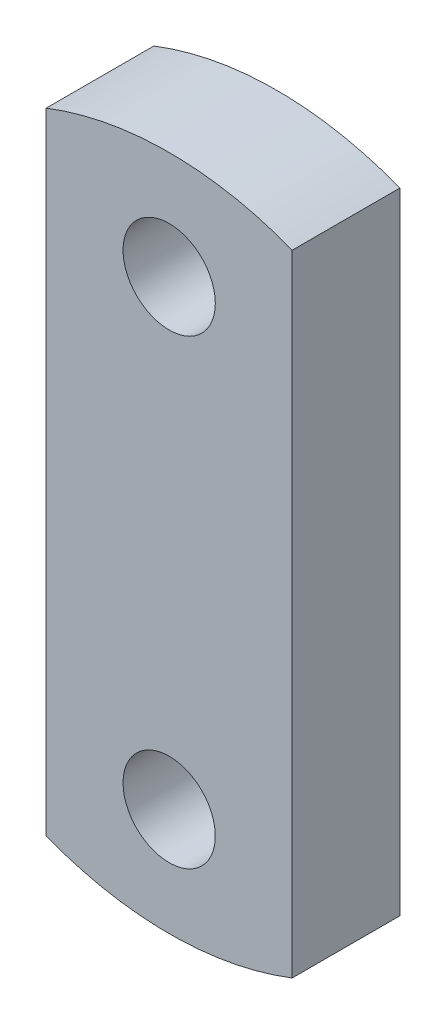
ISO-10303-21;
HEADER;
FILE_DESCRIPTION(('STEP AP214'),'2;1');
FILE_NAME('part.step','',(''),(''),'','','');
FILE_SCHEMA(('AUTOMOTIVE_DESIGN { 1 0 10303 214 1 1 1 1 }'));
ENDSEC;
DATA;
#1=APPLICATION_CONTEXT('core data for automotive mechanical design processes');
#2=APPLICATION_PROTOCOL_DEFINITION('international standard','automotive_design',2000,#1);
#3=PRODUCT_CONTEXT('',#1,'mechanical');
#4=PRODUCT('Part','Part','',(#3));
#5=PRODUCT_RELATED_PRODUCT_CATEGORY('part','',(#4));
#6=PRODUCT_DEFINITION_FORMATION('','',#4);
#7=PRODUCT_DEFINITION_CONTEXT('part definition',#1,'design');
#8=PRODUCT_DEFINITION('design','',#6,#7);
#9=PRODUCT_DEFINITION_SHAPE('','',#8);
#10=(LENGTH_UNIT() NAMED_UNIT(*) SI_UNIT(.MILLI.,.METRE.));
#11=(NAMED_UNIT(*) PLANE_ANGLE_UNIT() SI_UNIT($,.RADIAN.));
#12=(NAMED_UNIT(*) SI_UNIT($,.STERADIAN.) SOLID_ANGLE_UNIT());
#13=UNCERTAINTY_MEASURE_WITH_UNIT(LENGTH_MEASURE(1.E-05),#10,'distance_accuracy_value','');
#14=(GEOMETRIC_REPRESENTATION_CONTEXT(3) GLOBAL_UNCERTAINTY_ASSIGNED_CONTEXT((#13)) GLOBAL_UNIT_ASSIGNED_CONTEXT((#10,
#11,#12)) REPRESENTATION_CONTEXT('',''));
#15=CARTESIAN_POINT('',(0.,0.,0.));
#16=DIRECTION('',(0.,0.,1.));
#17=DIRECTION('',(1.,0.,0.));
#18=AXIS2_PLACEMENT_3D('',#15,#16,#17);
#19=CARTESIAN_POINT('',(0.,0.,17.5));
#20=DIRECTION('',(0.,0.,-1.));
#21=DIRECTION('',(-1.,0.,0.));
#22=AXIS2_PLACEMENT_3D('',#19,#20,#21);
#23=PLANE('',#22);
#24=CARTESIAN_POINT('',(0.,0.,17.5));
#25=DIRECTION('',(0.,0.,1.));
#26=DIRECTION('',(-1.,0.,0.));
#27=AXIS2_PLACEMENT_3D('',#24,#25,#26);
#28=CIRCLE('',#27,110.);
#29=CARTESIAN_POINT('',(40.,102.469507659596,17.5));
#30=VERTEX_POINT('',#29);
#31=CARTESIAN_POINT('',(-40.,102.469507659596,17.5));
#32=VERTEX_POINT('',#31);
#33=EDGE_CURVE('E93',#30,#32,#28,.T.);
#34=ORIENTED_EDGE('',*,*,#33,.T.);
#35=DIRECTION('',(0.,-1.,0.));
#36=VECTOR('',#35,1.);
#37=CARTESIAN_POINT('',(-40.,-102.469507659596,17.5));
#38=LINE('',#37,#36);
#39=CARTESIAN_POINT('',(-40.,-102.469507659596,17.5));
#40=VERTEX_POINT('',#39);
#41=EDGE_CURVE('E88',#32,#40,#38,.T.);
#42=ORIENTED_EDGE('',*,*,#41,.T.);
#43=CARTESIAN_POINT('',(0.,0.,17.5));
#44=DIRECTION('',(0.,0.,1.));
#45=DIRECTION('',(1.,0.,0.));
#46=AXIS2_PLACEMENT_3D('',#43,#44,#45);
#47=CIRCLE('',#46,110.);
#48=CARTESIAN_POINT('',(40.,-102.469507659596,17.5));
#49=VERTEX_POINT('',#48);
#50=EDGE_CURVE('E90',#40,#49,#47,.T.);
#51=ORIENTED_EDGE('',*,*,#50,.T.);
#52=DIRECTION('',(0.,1.,0.));
#53=VECTOR('',#52,1.);
#54=CARTESIAN_POINT('',(40.,-102.469507659596,17.5));
#55=LINE('',#54,#53);
#56=EDGE_CURVE('E57',#49,#30,#55,.T.);
#57=ORIENTED_EDGE('',*,*,#56,.T.);
#58=EDGE_LOOP('',(#34,#42,#51,#57));
#59=FACE_BOUND('',#58,.T.);
#60=CARTESIAN_POINT('',(0.,75.,17.5));
#61=DIRECTION('',(0.,0.,1.));
#62=DIRECTION('',(1.,0.,0.));
#63=AXIS2_PLACEMENT_3D('',#60,#61,#62);
#64=CIRCLE('',#63,15.);
#65=CARTESIAN_POINT('',(15.,75.,17.5));
#66=VERTEX_POINT('',#65);
#67=EDGE_CURVE('E106',#66,#66,#64,.T.);
#68=ORIENTED_EDGE('',*,*,#67,.F.);
#69=EDGE_LOOP('',(#68));
#70=FACE_BOUND('',#69,.T.);
#71=CARTESIAN_POINT('',(0.,-75.,17.5));
#72=DIRECTION('',(0.,0.,1.));
#73=DIRECTION('',(-1.,0.,0.));
#74=AXIS2_PLACEMENT_3D('',#71,#72,#73);
#75=CIRCLE('',#74,15.);
#76=CARTESIAN_POINT('',(-15.,-75.,17.5));
#77=VERTEX_POINT('',#76);
#78=EDGE_CURVE('E121',#77,#77,#75,.T.);
#79=ORIENTED_EDGE('',*,*,#78,.F.);
#80=EDGE_LOOP('',(#79));
#81=FACE_BOUND('',#80,.T.);
#82=ADVANCED_FACE('F39',(#59,#70,#81),#23,.F.);
#83=CARTESIAN_POINT('',(0.,0.,-17.5));
#84=DIRECTION('',(0.,0.,-1.));
#85=DIRECTION('',(-1.,0.,0.));
#86=AXIS2_PLACEMENT_3D('',#83,#84,#85);
#87=PLANE('',#86);
#88=CARTESIAN_POINT('',(0.,75.,-17.5));
#89=DIRECTION('',(0.,0.,1.));
#90=DIRECTION('',(1.,0.,0.));
#91=AXIS2_PLACEMENT_3D('',#88,#89,#90);
#92=CIRCLE('',#91,15.);
#93=CARTESIAN_POINT('',(15.,75.,-17.5));
#94=VERTEX_POINT('',#93);
#95=EDGE_CURVE('E119',#94,#94,#92,.T.);
#96=ORIENTED_EDGE('',*,*,#95,.T.);
#97=EDGE_LOOP('',(#96));
#98=FACE_BOUND('',#97,.T.);
#99=CARTESIAN_POINT('',(0.,0.,-17.5));
#100=DIRECTION('',(0.,0.,1.));
#101=DIRECTION('',(-1.,0.,0.));
#102=AXIS2_PLACEMENT_3D('',#99,#100,#101);
#103=CIRCLE('',#102,110.);
#104=CARTESIAN_POINT('',(40.,102.469507659596,-17.5));
#105=VERTEX_POINT('',#104);
#106=CARTESIAN_POINT('',(-40.,102.469507659596,-17.5));
#107=VERTEX_POINT('',#106);
#108=EDGE_CURVE('E103',#105,#107,#103,.T.);
#109=ORIENTED_EDGE('',*,*,#108,.F.);
#110=DIRECTION('',(0.,1.,0.));
#111=VECTOR('',#110,1.);
#112=CARTESIAN_POINT('',(40.,-102.469507659596,-17.5));
#113=LINE('',#112,#111);
#114=CARTESIAN_POINT('',(40.,-102.469507659596,-17.5));
#115=VERTEX_POINT('',#114);
#116=EDGE_CURVE('E76',#115,#105,#113,.T.);
#117=ORIENTED_EDGE('',*,*,#116,.F.);
#118=CARTESIAN_POINT('',(0.,0.,-17.5));
#119=DIRECTION('',(0.,0.,1.));
#120=DIRECTION('',(1.,0.,0.));
#121=AXIS2_PLACEMENT_3D('',#118,#119,#120);
#122=CIRCLE('',#121,110.);
#123=CARTESIAN_POINT('',(-40.,-102.469507659596,-17.5));
#124=VERTEX_POINT('',#123);
#125=EDGE_CURVE('E71',#124,#115,#122,.T.);
#126=ORIENTED_EDGE('',*,*,#125,.F.);
#127=DIRECTION('',(0.,-1.,0.));
#128=VECTOR('',#127,1.);
#129=CARTESIAN_POINT('',(-40.,-102.469507659596,-17.5));
#130=LINE('',#129,#128);
#131=EDGE_CURVE('E92',#107,#124,#130,.T.);
#132=ORIENTED_EDGE('',*,*,#131,.F.);
#133=EDGE_LOOP('',(#109,#117,#126,#132));
#134=FACE_BOUND('',#133,.T.);
#135=CARTESIAN_POINT('',(0.,-75.,-17.5));
#136=DIRECTION('',(0.,0.,1.));
#137=DIRECTION('',(-1.,0.,0.));
#138=AXIS2_PLACEMENT_3D('',#135,#136,#137);
#139=CIRCLE('',#138,15.);
#140=CARTESIAN_POINT('',(-15.,-75.,-17.5));
#141=VERTEX_POINT('',#140);
#142=EDGE_CURVE('E122',#141,#141,#139,.T.);
#143=ORIENTED_EDGE('',*,*,#142,.T.);
#144=EDGE_LOOP('',(#143));
#145=FACE_BOUND('',#144,.T.);
#146=ADVANCED_FACE('F111',(#98,#134,#145),#87,.T.);
#147=CARTESIAN_POINT('',(0.,0.,17.5));
#148=DIRECTION('',(0.,0.,-1.));
#149=DIRECTION('',(-1.,0.,0.));
#150=AXIS2_PLACEMENT_3D('',#147,#148,#149);
#151=CYLINDRICAL_SURFACE('',#150,110.);
#152=ORIENTED_EDGE('',*,*,#108,.T.);
#153=DIRECTION('',(0.,0.,-1.));
#154=VECTOR('',#153,1.);
#155=CARTESIAN_POINT('',(-40.,102.469507659596,17.5));
#156=LINE('',#155,#154);
#157=EDGE_CURVE('E11',#32,#107,#156,.T.);
#158=ORIENTED_EDGE('',*,*,#157,.F.);
#159=ORIENTED_EDGE('',*,*,#33,.F.);
#160=DIRECTION('',(0.,0.,-1.));
#161=VECTOR('',#160,1.);
#162=CARTESIAN_POINT('',(40.,102.469507659596,17.5));
#163=LINE('',#162,#161);
#164=EDGE_CURVE('E97',#30,#105,#163,.T.);
#165=ORIENTED_EDGE('',*,*,#164,.T.);
#166=EDGE_LOOP('',(#152,#158,#159,#165));
#167=FACE_BOUND('',#166,.T.);
#168=ADVANCED_FACE('F41',(#167),#151,.T.);
#169=CARTESIAN_POINT('',(-40.,-102.469507659596,17.5));
#170=DIRECTION('',(1.,0.,0.));
#171=DIRECTION('',(0.,0.,-1.));
#172=AXIS2_PLACEMENT_3D('',#169,#170,#171);
#173=PLANE('',#172);
#174=ORIENTED_EDGE('',*,*,#131,.T.);
#175=DIRECTION('',(0.,0.,-1.));
#176=VECTOR('',#175,1.);
#177=CARTESIAN_POINT('',(-40.,-102.469507659596,17.5));
#178=LINE('',#177,#176);
#179=EDGE_CURVE('E48',#40,#124,#178,.T.);
#180=ORIENTED_EDGE('',*,*,#179,.F.);
#181=ORIENTED_EDGE('',*,*,#41,.F.);
#182=ORIENTED_EDGE('',*,*,#157,.T.);
#183=EDGE_LOOP('',(#174,#180,#181,#182));
#184=FACE_BOUND('',#183,.T.);
#185=ADVANCED_FACE('F94',(#184),#173,.F.);
#186=CARTESIAN_POINT('',(0.,0.,17.5));
#187=DIRECTION('',(0.,0.,-1.));
#188=DIRECTION('',(-1.,0.,0.));
#189=AXIS2_PLACEMENT_3D('',#186,#187,#188);
#190=CYLINDRICAL_SURFACE('',#189,110.);
#191=ORIENTED_EDGE('',*,*,#125,.T.);
#192=DIRECTION('',(0.,0.,-1.));
#193=VECTOR('',#192,1.);
#194=CARTESIAN_POINT('',(40.,-102.469507659596,17.5));
#195=LINE('',#194,#193);
#196=EDGE_CURVE('E96',#49,#115,#195,.T.);
#197=ORIENTED_EDGE('',*,*,#196,.F.);
#198=ORIENTED_EDGE('',*,*,#50,.F.);
#199=ORIENTED_EDGE('',*,*,#179,.T.);
#200=EDGE_LOOP('',(#191,#197,#198,#199));
#201=FACE_BOUND('',#200,.T.);
#202=ADVANCED_FACE('F100',(#201),#190,.T.);
#203=CARTESIAN_POINT('',(40.,-102.469507659596,17.5));
#204=DIRECTION('',(-1.,0.,0.));
#205=DIRECTION('',(0.,0.,1.));
#206=AXIS2_PLACEMENT_3D('',#203,#204,#205);
#207=PLANE('',#206);
#208=ORIENTED_EDGE('',*,*,#116,.T.);
#209=ORIENTED_EDGE('',*,*,#164,.F.);
#210=ORIENTED_EDGE('',*,*,#56,.F.);
#211=ORIENTED_EDGE('',*,*,#196,.T.);
#212=EDGE_LOOP('',(#208,#209,#210,#211));
#213=FACE_BOUND('',#212,.T.);
#214=ADVANCED_FACE('F112',(#213),#207,.F.);
#215=CARTESIAN_POINT('',(0.,75.,17.5));
#216=DIRECTION('',(0.,0.,-1.));
#217=DIRECTION('',(-1.,0.,0.));
#218=AXIS2_PLACEMENT_3D('',#215,#216,#217);
#219=CYLINDRICAL_SURFACE('',#218,15.);
#220=ORIENTED_EDGE('',*,*,#67,.T.);
#221=EDGE_LOOP('',(#220));
#222=FACE_BOUND('',#221,.T.);
#223=ORIENTED_EDGE('',*,*,#95,.F.);
#224=EDGE_LOOP('',(#223));
#225=FACE_BOUND('',#224,.T.);
#226=ADVANCED_FACE('F143',(#222,#225),#219,.F.);
#227=CARTESIAN_POINT('',(0.,-75.,17.5));
#228=DIRECTION('',(0.,0.,-1.));
#229=DIRECTION('',(-1.,0.,0.));
#230=AXIS2_PLACEMENT_3D('',#227,#228,#229);
#231=CYLINDRICAL_SURFACE('',#230,15.);
#232=ORIENTED_EDGE('',*,*,#78,.T.);
#233=EDGE_LOOP('',(#232));
#234=FACE_BOUND('',#233,.T.);
#235=ORIENTED_EDGE('',*,*,#142,.F.);
#236=EDGE_LOOP('',(#235));
#237=FACE_BOUND('',#236,.T.);
#238=ADVANCED_FACE('F128',(#234,#237),#231,.F.);
#239=CLOSED_SHELL('',(#82,#146,#168,#185,#202,#214,#226,#238));
#240=MANIFOLD_SOLID_BREP('B2',#239);
#241=ADVANCED_BREP_SHAPE_REPRESENTATION('',(#18,#240),#14);
#242=SHAPE_DEFINITION_REPRESENTATION(#9,#241);
ENDSEC;
END-ISO-10303-21;
